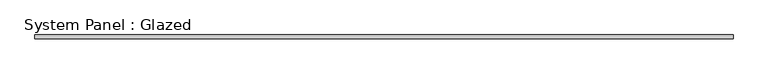
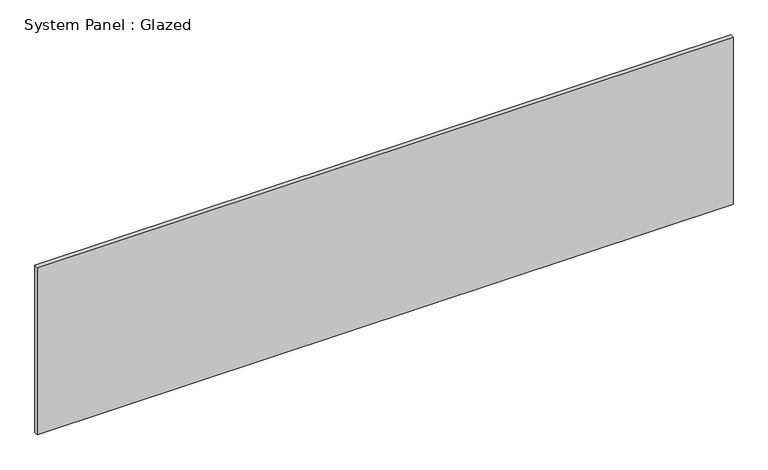
"""IFC4 building model written with IfcOpenShell, lengths in millimetres: plate geometry, System Panel : Glazed."""

from ifc_helpers import new_model, si_unit, origin, origin_with_axes, place, context, project, spatial, polyline, outline, extrude, source, transform, mapped, element, save


def system_panel_glazed_dc8eac37(model_context):
    return source(origin(), model_context, "Body", "SweptSolid", [
        extrude(outline(polyline([(2277.5162995, 19.05), (-2277.5162995, 19.05), (-2277.5162995, 44.45), (2277.5162995, 44.45), (2277.5162995, 19.05)])), origin_with_axes(), (0.0, 0.0, 1.0), 1155.7),
    ])


if __name__ == "__main__":
    model = new_model("IFC4")
    model_context = context("Model", 3, world=origin())
    ifc_project = project(units=[si_unit("LENGTHUNIT", "METRE", prefix="MILLI")], contexts=[model_context])
    site = spatial("IfcSite", under=ifc_project)
    building = spatial("IfcBuilding", under=site)
    placement = place(None, origin())
    system_panel_glazed_shape = system_panel_glazed_dc8eac37(model_context)
    element("IfcPlate", 1, ObjectType="System Panel : Glazed", at=placement, inside=building, context=model_context, shape_type="MappedRepresentation", body=[
        mapped(system_panel_glazed_shape, transform((0.0, 0.0, 0.0), x_axis=(1.0, 0.0, 0.0), y_axis=(0.0, 1.0, 0.0), z_axis=(0.0, 0.0, 1.0))),
    ])
    save(model, "model.ifc")

# Revit data of these elements
# Type "System Panel : Glazed"
#   Construction Type Id = "GSP4R"
#   Analytic Construction = "1/8 in Pilkington single glazing"
#   Visual Light Transmittance = 0.9
#   Solar Heat Gain Coefficient = 0.86
#   Heat Transfer Coefficient (U) = 1.18115 BTU/(h·ft²·°F)
# Element 1 (IfcPlate, "System Panel : Glazed")
#   Materials on its faces: "Glass"
# Materials
#   "Glass": class "Glass", colour RGB 0 128 192, transparency 0.75, Description = "Soda Lime Glass", Cost = 0
